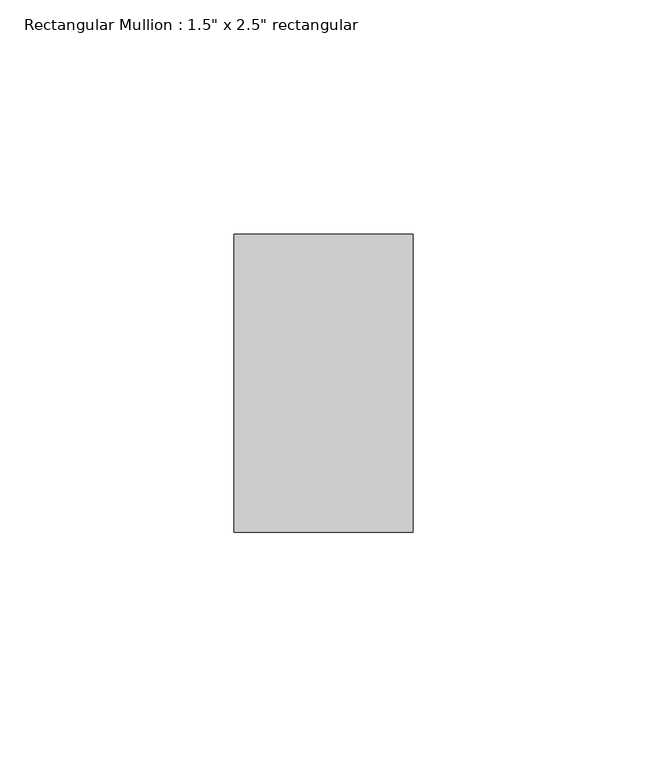
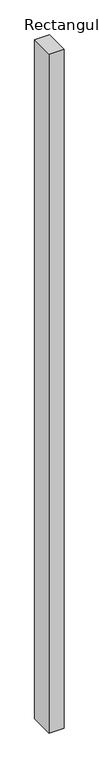
"""IFC4 building model written with IfcOpenShell, lengths in millimetres: member geometry."""

from ifc_helpers import new_model, si_unit, frame, origin, place, context, project, spatial, polyline, outline, extrude, source, transform, mapped, element, save


def member_b71d7755(model_context):
    return source(origin(), model_context, "Body", "SweptSolid", [
        extrude(outline(polyline([(0.0, 31.75), (0.0, -31.75), (-38.1, -31.75), (-38.1, 31.75), (0.0, 31.75)])), frame((0.0, 0.0, -1828.8), z_axis=(0.0, 0.0, 1.0), x_axis=(1.0, 0.0, 0.0)), (0.0, 0.0, 1.0), 1828.8),
    ])


if __name__ == "__main__":
    model = new_model("IFC4")
    model_context = context("Model", 3, world=origin())
    ifc_project = project(units=[si_unit("LENGTHUNIT", "METRE", prefix="MILLI")], contexts=[model_context])
    site = spatial("IfcSite", under=ifc_project)
    building = spatial("IfcBuilding", under=site)
    placement = place(None, origin())
    member_shape = member_b71d7755(model_context)
    element("IfcMember", 1, ObjectType="Rectangular Mullion : 1.5\" x 2.5\" rectangular", at=placement, inside=building, context=model_context, shape_type="MappedRepresentation", body=[
        mapped(member_shape, transform((0.0, 0.0, 0.0), x_axis=(1.0, 0.0, 0.0), y_axis=(0.0, 1.0, 0.0), z_axis=(0.0, 0.0, 1.0))),
    ])
    save(model, "model.ifc")

# Revit data of these elements
# Type "Rectangular Mullion : 1.5\" x 2.5\" rectangular"
#   built-in parameter 1007304 = 0.208333 (stored number, unit not read)
#   built-in parameter 1007301 = 0.0625 (stored number, unit not read)
#   built-in parameter 1007300 = 0.0625 (stored number, unit not read)
# Element 1 (IfcMember, "Rectangular Mullion : 1.5\" x 2.5\" rectangular")
#   Materials on its faces: "Aluminum"
# Materials
#   "Aluminum": class "Metal", colour RGB 247 247 247, transparency 0, Description = "Aluminum 6061", Cost = 0
